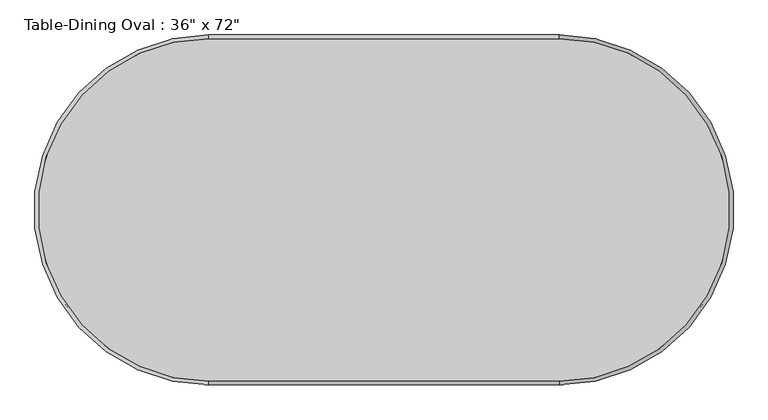
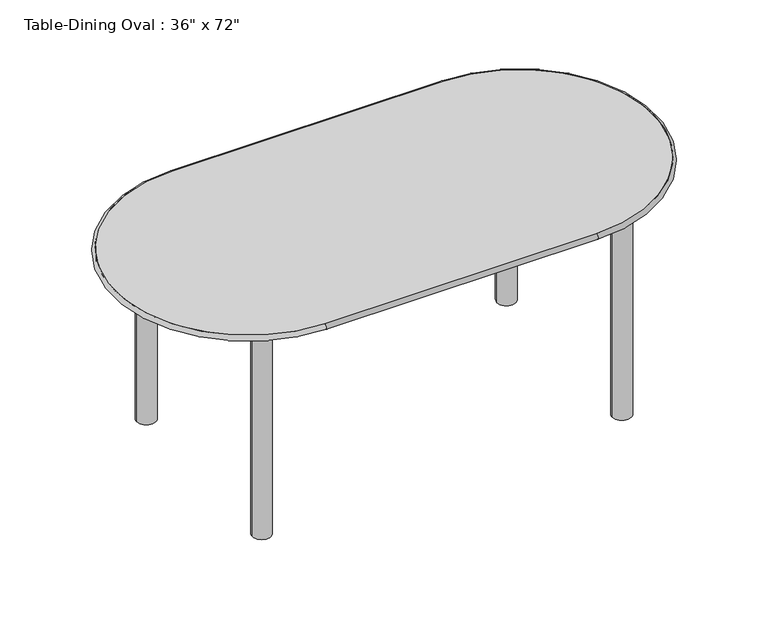
"""IFC4 building model written with IfcOpenShell, lengths in millimetres: furniture geometry."""

from ifc_helpers import new_model, si_unit, point, frame, frame_2d, origin, origin_with_axes, place, context, project, spatial, polyline, circle_curve, ellipse_curve, trimmed, segment, composite_curve, outline, extrude, source, transform, mapped, element, save
from ifc_brep_helpers import plane_surface, cylinder_surface, revolved_surface, advanced_brep


def furniture_2c34a4f9(model_context):
    return source(origin(), model_context, "Body", "SolidModel", [
        advanced_brep(
        [(-859.0196721, -805.7733607, 762.0), (-859.0196721, -805.7733607, 742.95), (55.3803279, -805.7733607, 742.95), (55.3803279, -805.7733607, 762.0), (55.3803279, 89.5766393, 762.0), (55.3803279, 89.5766393, 742.95), (-859.0196721, 89.5766393, 742.95), (-859.0196721, 89.5766393, 762.0)],
        [
            (0, 1, circle_curve(frame((-859.0196721, -805.7733607, 752.475), z_axis=(1.0, 0.0, 0.0), x_axis=(0.0, 1.0, 0.0)), 9.525)),
            (1, 2),
            (2, 3, circle_curve(frame((55.3803279, -805.7733607, 752.475), z_axis=(-1.0, 0.0, 0.0), x_axis=(0.0, 1.0, 0.0)), 9.525)),
            (3, 0),
            (1, 0),
            (3, 2),
            (4, 3, circle_curve(frame((55.3803279, -358.0983607, 762.0), z_axis=(0.0, 0.0, -1.0), x_axis=(0.0, -1.0, 0.0)), 447.675)),
            (2, 5, circle_curve(frame((55.3803279, -358.0983607, 742.95), z_axis=(0.0, 0.0, 1.0), x_axis=(0.0, -1.0, 0.0)), 447.675)),
            (5, 4, circle_curve(frame((55.3803279, 89.5766393, 752.475), z_axis=(1.0, 0.0, 0.0), x_axis=(0.0, -1.0, 0.0)), 9.525)),
            (4, 5),
            (5, 6),
            (6, 7, circle_curve(frame((-859.0196721, 89.5766393, 752.475), z_axis=(1.0, 0.0, 0.0), x_axis=(0.0, -1.0, 0.0)), 9.525)),
            (7, 4),
            (7, 6),
            (0, 7, circle_curve(frame((-859.0196721, -358.0983607, 762.0), z_axis=(0.0, 0.0, -1.0), x_axis=(0.0, 1.0, 0.0)), 447.675)),
            (6, 1, circle_curve(frame((-859.0196721, -358.0983607, 742.95), z_axis=(0.0, 0.0, 1.0), x_axis=(0.0, 1.0, 0.0)), 447.675)),
        ],
        [
            cylinder_surface(frame((-859.0196721, -805.7733607, 752.475), z_axis=(-1.0, 0.0, 0.0), x_axis=(0.0, 1.0, 0.0)), 9.525),
            plane_surface(frame((-859.0196721, -805.7733607, 762.0), z_axis=(0.0, 1.0, 0.0), x_axis=(1.0, 0.0, 0.0))),
            revolved_surface(trimmed(ellipse_curve(frame((55.3803279, -805.7733607, 752.475), z_axis=(-1.0, 0.0, 0.0), x_axis=(0.0, 1.0, 0.0)), 9.525, 9.525), [point((55.3803279, -805.7733607, 742.95))], [point((55.3803279, -805.7733607, 762.0))], True, "CARTESIAN"), (55.3803279, -358.0983607, 0.0), (0.0, 0.0, 1.0)),
            revolved_surface(polyline([(55.3803279, -805.7733607, 762.0), (55.3803279, -805.7733607, 742.95)]), (55.3803279, -358.0983607, 0.0), (0.0, 0.0, 1.0)),
            cylinder_surface(frame((55.3803279, 89.5766393, 752.475), z_axis=(1.0, 0.0, 0.0), x_axis=(0.0, -1.0, 0.0)), 9.525),
            plane_surface(frame((55.3803279, 89.5766393, 762.0), z_axis=(0.0, -1.0, 0.0), x_axis=(-1.0, 0.0, 0.0))),
            revolved_surface(trimmed(ellipse_curve(frame((-859.0196721, 89.5766393, 752.475), z_axis=(1.0, 0.0, 0.0), x_axis=(0.0, -1.0, 0.0)), 9.525, 9.525), [point((-859.0196721, 89.5766393, 742.95))], [point((-859.0196721, 89.5766393, 762.0))], True, "CARTESIAN"), (-859.0196721, -358.0983607, 0.0), (0.0, 0.0, 1.0)),
            revolved_surface(polyline([(-859.0196721, 89.57663930000001, 762.0), (-859.0196721, 89.57663930000001, 742.95)]), (-859.0196721, -358.0983607, 0.0), (0.0, 0.0, 1.0)),
        ],
        [
            (0, [[1, 2, 3, 4]]),
            (1, [[5, -4, 6, -2]]),
            (2, [[7, -3, 8, 9]]),
            (3, [[-8, -6, -7, 10]]),
            (4, [[-9, 11, 12, 13]]),
            (5, [[-10, -13, 14, -11]]),
            (6, [[15, -12, 16, -1]]),
            (7, [[-16, -14, -15, -5]]),
        ],
    ),
        extrude(outline(composite_curve([segment(trimmed(circle_curve(frame_2d((-1008.2446721, -21.5483607)), 31.75), [point((-1039.9946721, -21.5483607))], [point((-976.4946721, -21.5483607))], False, "CARTESIAN"), True, "CONTINUOUS"), segment(trimmed(circle_curve(frame_2d((-1008.2446721, -21.5483607)), 31.75), [point((-976.4946721, -21.5483607))], [point((-1039.9946721, -21.5483607))], False, "CARTESIAN"), True, "CONTINUOUS")], self_intersect=False)), origin_with_axes(), (0.0, 0.0, 1.0), 742.95),
        extrude(outline(composite_curve([segment(trimmed(circle_curve(frame_2d((-1008.2446721, -694.6483607)), 31.75), [point((-1039.9946721, -694.6483607))], [point((-976.4946721, -694.6483607))], False, "CARTESIAN"), True, "CONTINUOUS"), segment(trimmed(circle_curve(frame_2d((-1008.2446721, -694.6483607)), 31.75), [point((-976.4946721, -694.6483607))], [point((-1039.9946721, -694.6483607))], False, "CARTESIAN"), True, "CONTINUOUS")], self_intersect=False)), origin_with_axes(), (0.0, 0.0, 1.0), 742.95),
        extrude(outline(composite_curve([segment(trimmed(circle_curve(frame_2d((204.6053279, -21.5483607)), 31.75), [point((172.8553279, -21.5483607))], [point((236.3553279, -21.5483607))], False, "CARTESIAN"), True, "CONTINUOUS"), segment(trimmed(circle_curve(frame_2d((204.6053279, -21.5483607)), 31.75), [point((236.3553279, -21.5483607))], [point((172.8553279, -21.5483607))], False, "CARTESIAN"), True, "CONTINUOUS")], self_intersect=False)), origin_with_axes(), (0.0, 0.0, 1.0), 742.95),
        extrude(outline(composite_curve([segment(trimmed(circle_curve(frame_2d((204.6053279, -694.6483607)), 31.75), [point((172.8553279, -694.6483607))], [point((236.3553279, -694.6483607))], False, "CARTESIAN"), True, "CONTINUOUS"), segment(trimmed(circle_curve(frame_2d((204.6053279, -694.6483607)), 31.75), [point((236.3553279, -694.6483607))], [point((172.8553279, -694.6483607))], False, "CARTESIAN"), True, "CONTINUOUS")], self_intersect=False)), origin_with_axes(), (0.0, 0.0, 1.0), 742.95),
        extrude(outline(polyline([(223.6553279, -2.4983607), (223.6553279, -713.6983607), (-1027.2946721, -713.6983607), (-1027.2946721, -2.4983607), (223.6553279, -2.4983607)]), holes=[polyline([(204.6053279, -21.5483607), (-1008.2446721, -21.5483607), (-1008.2446721, -694.6483607), (204.6053279, -694.6483607), (204.6053279, -21.5483607)])]), frame((0.0, 0.0, 692.15), z_axis=(0.0, 0.0, 1.0), x_axis=(1.0, 0.0, 0.0)), (0.0, 0.0, 1.0), 50.8),
        extrude(outline(composite_curve([segment(polyline([(-859.0196721, 89.5766393), (55.3803279, 89.5766393)]), True, "CONTINUOUS"), segment(trimmed(circle_curve(frame_2d((55.3803279, -358.0983607)), 447.675), [point((55.3803279, 89.5766393))], [point((503.0553279, -358.0983607))], False, "CARTESIAN"), True, "CONTINUOUS"), segment(trimmed(circle_curve(frame_2d((55.3803279, -358.0983607)), 447.675), [point((503.0553279, -358.0983607))], [point((55.3803279, -805.7733607))], False, "CARTESIAN"), True, "CONTINUOUS"), segment(polyline([(55.3803279, -805.7733607), (-859.0196721, -805.7733607)]), True, "CONTINUOUS"), segment(trimmed(circle_curve(frame_2d((-859.0196721, -358.0983607)), 447.675), [point((-859.0196721, -805.7733607))], [point((-1306.6946721, -358.0983607))], False, "CARTESIAN"), True, "CONTINUOUS"), segment(trimmed(circle_curve(frame_2d((-859.0196721, -358.0983607)), 447.675), [point((-1306.6946721, -358.0983607))], [point((-859.0196721, 89.5766393))], False, "CARTESIAN"), True, "CONTINUOUS")], self_intersect=False)), frame((0.0, 0.0, 742.95), z_axis=(0.0, 0.0, 1.0), x_axis=(1.0, 0.0, 0.0)), (0.0, 0.0, 1.0), 19.05),
    ])


if __name__ == "__main__":
    model = new_model("IFC4")
    model_context = context("Model", 3, world=origin())
    ifc_project = project(units=[si_unit("LENGTHUNIT", "METRE", prefix="MILLI")], contexts=[model_context])
    site = spatial("IfcSite", under=ifc_project)
    building = spatial("IfcBuilding", under=site)
    placement = place(None, origin())
    furniture_shape = furniture_2c34a4f9(model_context)
    element("IfcFurniture", 1, ObjectType="Table-Dining Oval : 36\" x 72\"", at=placement, inside=building, context=model_context, shape_type="MappedRepresentation", body=[
        mapped(furniture_shape, transform((0.0, 0.0, 0.0), x_axis=(1.0, 0.0, 0.0), y_axis=(0.0, 1.0, 0.0), z_axis=(0.0, 0.0, 1.0))),
    ])
    save(model, "model.ifc")

# Revit data of these elements
# Type "Table-Dining Oval : 36\" x 72\""
#   Assembly Code = "E2020200"
#   Length = 6' - 0"
#   Width = 3' - 0"
#   Base Material = Steel, Chrome Plated
#   Top Material = Glass - Clear, Grey
#   Default Elevation = 0
#   Description = (empty or 0)
# Element 1 (IfcFurniture, "Table-Dining Oval : 36\" x 72\"")
#   Materials on its faces: "Steel, Chrome Plated", "Glass - Clear, Grey"
# Materials
#   "Steel, Chrome Plated": class "Metal", colour RGB 17 17 17, transparency 0, Description = "Chromiuim plated steel", Cost = 0
#   "Glass - Clear, Grey": class "Glass", colour RGB 252 255 255, transparency 0.64
